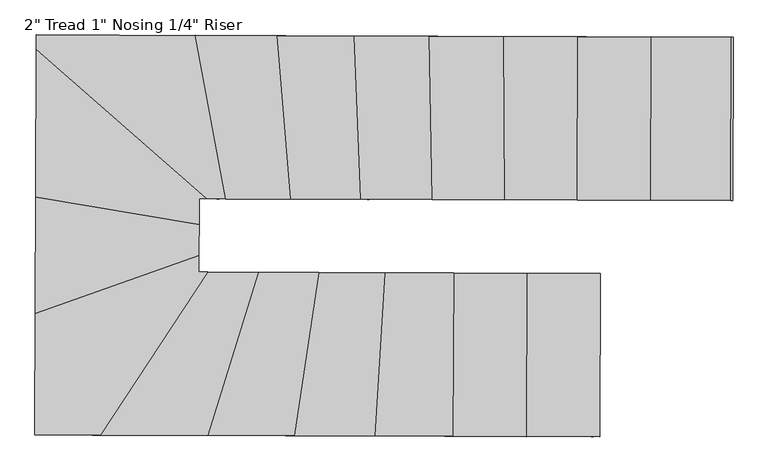
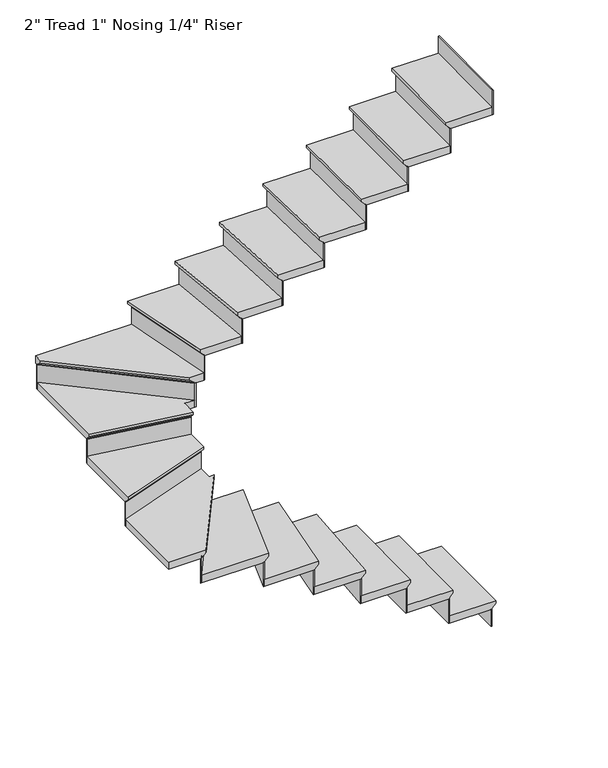
"""IFC4 building model written with IfcOpenShell, lengths in millimetres: stair flight geometry."""

from ifc_helpers import new_model, si_unit, origin, place, context, project, spatial, faceted_brep, source, transform, mapped, element, save


def stair_flight_0ba6b5c4(model_context):
    return source(origin(), model_context, "Body", "Brep", [
        faceted_brep([(-2339.9228929, -4204.0248458, 150.2833333), (-2339.9228929, -4204.0248458, 169.3333333), (-2342.0274141, -4826.0015756, 169.3333333), (-2342.0274141, -4826.0015756, 150.2833333), (-2365.3227475, -4203.9389029, 124.8833333), (-2367.4272687, -4825.9156326, 124.8833333), (-2644.7211481, -4202.9935301, 169.3333333), (-2646.8256693, -4824.9702599, 169.3333333), (-2367.4272687, -4825.9156326, 118.5333333), (-2646.8256693, -4824.9702599, 118.5333333), (-2644.7211481, -4202.9935301, 118.5333333), (-2365.3227475, -4203.9389029, 118.5333333)], [[[0, 1, 2, 3]], [[4, 0, 3, 5]], [[2, 1, 6, 7]], [[8, 9, 10, 11]], [[2, 7, 9, 8, 5, 3]], [[8, 11, 4, 5]], [[6, 1, 0, 4, 11, 10]], [[7, 6, 10, 9]]]),
        faceted_brep([(-2365.3227475, -4203.9389029, 118.5333333), (-2365.3227475, -4203.9389029, 0.0), (-2371.6727112, -4203.9174171, 0.0), (-2371.6727112, -4203.9174171, 118.5333333), (-2367.4272687, -4825.9156326, 118.5333333), (-2373.7772323, -4825.8941469, 118.5333333), (-2373.7772323, -4825.8941469, 0.0), (-2367.4272687, -4825.9156326, 0.0)], [[[0, 1, 2, 3]], [[4, 5, 6, 7]], [[1, 0, 4, 7]], [[2, 1, 7, 6]], [[3, 2, 6, 5]], [[0, 3, 5, 4]]]),
        faceted_brep([(-2644.7211481, -4202.9935301, 287.8666667), (-2644.7211481, -4202.9935301, 118.5333333), (-2651.0711118, -4202.9720444, 118.5333333), (-2651.0711118, -4202.9720444, 287.8666667), (-2646.8256693, -4824.9702599, 287.8666667), (-2653.175633, -4824.9487741, 287.8666667), (-2653.175633, -4824.9487741, 118.5333333), (-2646.8256693, -4824.9702599, 118.5333333)], [[[0, 1, 2, 3]], [[4, 5, 6, 7]], [[1, 0, 4, 7]], [[2, 1, 7, 6]], [[3, 2, 6, 5]], [[0, 3, 5, 4]]]),
        faceted_brep([(-2621.4258147, -4825.0562028, 338.6666667), (-2619.3212935, -4203.0794731, 338.6666667), (-2924.1195488, -4202.0481574, 338.6666667), (-2926.2240699, -4824.0248871, 338.6666667), (-2646.8256693, -4824.9702599, 287.8666667), (-2926.2240699, -4824.0248871, 287.8666667), (-2924.1195488, -4202.0481574, 287.8666667), (-2644.7211481, -4202.9935301, 287.8666667), (-2646.8256693, -4824.9702599, 294.2166667), (-2621.4258147, -4825.0562028, 319.6166667), (-2644.7211481, -4202.9935301, 294.2166667), (-2619.3212935, -4203.0794731, 319.6166667)], [[[0, 1, 2, 3]], [[4, 5, 6, 7]], [[0, 3, 5, 4, 8, 9]], [[4, 7, 10, 8]], [[2, 1, 11, 10, 7, 6]], [[3, 2, 6, 5]], [[11, 1, 0, 9]], [[10, 11, 9, 8]]]),
        faceted_brep([(-2924.1195488, -4202.0481574, 457.2), (-2924.1195488, -4202.0481574, 287.8666667), (-2930.4695124, -4202.0266716, 287.8666667), (-2930.4695124, -4202.0266716, 457.2), (-2926.2240699, -4824.0248871, 457.2), (-2932.5740336, -4824.0034014, 457.2), (-2932.5740336, -4824.0034014, 287.8666667), (-2926.2240699, -4824.0248871, 287.8666667)], [[[0, 1, 2, 3]], [[4, 5, 6, 7]], [[1, 0, 4, 7]], [[2, 1, 7, 6]], [[3, 2, 6, 5]], [[0, 3, 5, 4]]]),
        faceted_brep([(-2900.8242153, -4824.1108301, 508.0), (-2898.7196941, -4202.1341003, 508.0), (-3185.4282049, -4201.1639931, 508.0), (-3223.7984946, -4823.0180139, 508.0), (-2926.2240699, -4824.0248871, 457.2), (-3223.7984946, -4823.0180139, 457.2), (-3185.4282049, -4201.1639931, 457.2), (-2924.1195488, -4202.0481574, 457.2), (-2926.2240699, -4824.0248871, 463.55), (-2900.8242153, -4824.1108301, 488.95), (-2924.1195488, -4202.0481574, 463.55), (-2898.7196941, -4202.1341003, 488.95)], [[[0, 1, 2, 3]], [[4, 5, 6, 7]], [[0, 3, 5, 4, 8, 9]], [[4, 7, 10, 8]], [[2, 1, 11, 10, 7, 6]], [[3, 2, 6, 5]], [[11, 1, 0, 9]], [[10, 11, 9, 8]]]),
        faceted_brep([(-3185.4282049, -4201.1639931, 626.5333333), (-3185.4282049, -4201.1639931, 457.2), (-3191.7889535, -4201.1424708, 457.2), (-3191.7889535, -4201.1424708, 626.5333333), (-3223.7984946, -4823.0180139, 626.5333333), (-3230.1592432, -4822.9964917, 626.5333333), (-3230.1592432, -4822.9964917, 457.2), (-3223.7984946, -4823.0180139, 457.2)], [[[0, 1, 2, 3]], [[4, 5, 6, 7]], [[1, 0, 4, 7]], [[2, 1, 7, 6]], [[3, 2, 6, 5]], [[0, 3, 5, 4]]]),
        faceted_brep([(-3198.3555003, -4823.1041029, 677.3333333), (-3159.9852105, -4201.250082, 677.3333333), (-3437.1491731, -4200.3122697, 677.3333333), (-3531.3418182, -4821.97741, 677.3333333), (-3223.7984946, -4823.0180139, 626.5333333), (-3531.3418182, -4821.97741, 626.5333333), (-3437.1491731, -4200.3122697, 626.5333333), (-3185.4282049, -4201.1639931, 626.5333333), (-3223.7984946, -4823.0180139, 632.8833333), (-3198.3555003, -4823.1041029, 658.2833333), (-3185.4282049, -4201.1639931, 632.8833333), (-3159.9852105, -4201.250082, 658.2833333)], [[[0, 1, 2, 3]], [[4, 5, 6, 7]], [[0, 3, 5, 4, 8, 9]], [[4, 7, 10, 8]], [[2, 1, 11, 10, 7, 6]], [[3, 2, 6, 5]], [[11, 1, 0, 9]], [[10, 11, 9, 8]]]),
        faceted_brep([(-3437.1491731, -4200.3122697, 795.8666667), (-3437.1491731, -4200.3122697, 626.5333333), (-3443.568358, -4200.2905498, 626.5333333), (-3443.568358, -4200.2905498, 795.8666667), (-3531.3418182, -4821.97741, 795.8666667), (-3537.7610031, -4821.95569, 795.8666667), (-3537.7610031, -4821.95569, 626.5333333), (-3531.3418182, -4821.97741, 626.5333333)], [[[0, 1, 2, 3]], [[4, 5, 6, 7]], [[1, 0, 4, 7]], [[2, 1, 7, 6]], [[3, 2, 6, 5]], [[0, 3, 5, 4]]]),
        faceted_brep([(-3505.6650785, -4822.0642898, 846.6666667), (-3411.4724335, -4200.3991496, 846.6666667), (-3668.9000376, -4199.5281172, 846.6666667), (-3860.1305452, -4820.8649201, 846.6666667), (-3531.3418182, -4821.97741, 795.8666667), (-3860.1305452, -4820.8649201, 795.8666667), (-3668.9000376, -4199.5281172, 795.8666667), (-3437.1491731, -4200.3122697, 795.8666667), (-3531.3418182, -4821.97741, 802.2166667), (-3505.6650785, -4822.0642898, 827.6166667), (-3437.1491731, -4200.3122697, 802.2166667), (-3411.4724335, -4200.3991496, 827.6166667)], [[[0, 1, 2, 3]], [[4, 5, 6, 7]], [[0, 3, 5, 4, 8, 9]], [[4, 7, 10, 8]], [[2, 1, 11, 10, 7, 6]], [[3, 2, 6, 5]], [[11, 1, 0, 9]], [[10, 11, 9, 8]]]),
        faceted_brep([(-3668.9000376, -4199.5281172, 965.2), (-3668.9000376, -4199.5281172, 795.8666667), (-3675.5370713, -4199.5056601, 795.8666667), (-3675.5370713, -4199.5056601, 965.2), (-3860.1305452, -4820.8649201, 965.2), (-3866.7675788, -4820.842463, 965.2), (-3866.7675788, -4820.842463, 795.8666667), (-3860.1305452, -4820.8649201, 795.8666667)], [[[0, 1, 2, 3]], [[4, 5, 6, 7]], [[1, 0, 4, 7]], [[2, 1, 7, 6]], [[3, 2, 6, 5]], [[0, 3, 5, 4]]]),
        faceted_brep([(-3833.5824104, -4820.9547484, 1016.0), (-3642.3519028, -4199.6179455, 1016.0), (-3864.4957991, -4198.8662992, 1016.0), (-4274.0422035, -4819.4644081, 1016.0), (-3860.1305452, -4820.8649201, 965.2), (-4274.0422035, -4819.4644081, 965.2), (-3864.4957991, -4198.8662992, 965.2), (-3668.9000376, -4199.5281172, 965.2), (-3860.1305452, -4820.8649201, 971.55), (-3833.5824104, -4820.9547484, 996.95), (-3668.9000376, -4199.5281172, 971.55), (-3642.3519028, -4199.6179455, 996.95)], [[[0, 1, 2, 3]], [[4, 5, 6, 7]], [[0, 3, 5, 4, 8, 9]], [[4, 7, 10, 8]], [[2, 1, 11, 10, 7, 6]], [[3, 2, 6, 5]], [[11, 1, 0, 9]], [[10, 11, 9, 8]]]),
        faceted_brep([(-3864.4957991, -4198.8662992, 1134.5333333), (-3864.4957991, -4198.8662992, 965.2), (-3872.0869257, -4198.8406138, 965.2), (-3872.0869257, -4198.8406138, 1134.5333333), (-4274.0422035, -4819.4644081, 1134.5333333), (-4281.6333301, -4819.4387227, 1134.5333333), (-4281.6333301, -4819.4387227, 965.2), (-4274.0422035, -4819.4644081, 965.2)], [[[0, 1, 2, 3]], [[4, 5, 6, 7]], [[1, 0, 4, 7]], [[2, 1, 7, 6]], [[3, 2, 6, 5]], [[0, 3, 5, 4]]]),
        faceted_brep([(-4490.0684734, -4328.5349965, 1185.3333333), (-4491.7270905, -4818.7278493, 1185.3333333), (-4243.677697, -4819.5671495, 1185.3333333), (-3834.1312926, -4198.9690405, 1185.3333333), (-3867.6458395, -4198.8556407, 1185.3333333), (-3867.338948, -4108.1559559, 1185.3333333), (-4491.7270905, -4818.7278493, 1134.5333333), (-4490.0684734, -4328.5349965, 1134.5333333), (-3867.338948, -4108.1559559, 1134.5333333), (-3867.6458395, -4198.8556407, 1134.5333333), (-3864.4957991, -4198.8662992, 1134.5333333), (-4274.0422035, -4819.4644081, 1134.5333333), (-4274.0422035, -4819.4644081, 1140.8833333), (-4243.677697, -4819.5671495, 1166.2833333), (-3864.4957991, -4198.8662992, 1140.8833333), (-3834.1312926, -4198.9690405, 1166.2833333)], [[[0, 1, 2, 3, 4, 5]], [[6, 7, 8, 9, 10, 11]], [[1, 0, 7, 6]], [[2, 1, 6, 11, 12, 13]], [[11, 10, 14, 12]], [[4, 3, 15, 14, 10, 9]], [[5, 4, 9, 8]], [[0, 5, 8, 7]], [[15, 3, 2, 13]], [[14, 15, 13, 12]]]),
        faceted_brep([(-3867.338948, -4108.1559559, 1303.8666667), (-3867.338948, -4108.1559559, 1134.5333333), (-3867.316129, -4101.4119712, 1134.5333333), (-3867.316129, -4101.4119712, 1303.8666667), (-4490.0684734, -4328.5349965, 1303.8666667), (-4490.0456544, -4321.7910118, 1303.8666667), (-4490.0456544, -4321.7910118, 1134.5333333), (-4490.0684734, -4328.5349965, 1134.5333333)], [[[0, 1, 2, 3]], [[4, 5, 6, 7]], [[1, 0, 4, 7]], [[2, 1, 7, 6]], [[3, 2, 6, 5]], [[0, 3, 5, 4]]]),
        faceted_brep([(-4490.1597492, -4355.5109354, 1354.6666667), (-3867.4302238, -4135.1318948, 1354.6666667), (-3866.9449143, -3991.702012, 1354.6666667), (-4488.5718319, -3886.2129338, 1354.6666667), (-4490.0684734, -4328.5349965, 1303.8666667), (-4488.5718319, -3886.2129338, 1303.8666667), (-3866.9449143, -3991.702012, 1303.8666667), (-3867.338948, -4108.1559559, 1303.8666667), (-4490.0684734, -4328.5349965, 1310.2166667), (-4490.1597492, -4355.5109354, 1335.6166667), (-3867.338948, -4108.1559559, 1310.2166667), (-3867.4302238, -4135.1318948, 1335.6166667)], [[[0, 1, 2, 3]], [[4, 5, 6, 7]], [[0, 3, 5, 4, 8, 9]], [[4, 7, 10, 8]], [[3, 2, 6, 5]], [[11, 1, 0, 9]], [[10, 11, 9, 8]], [[2, 1, 11, 10, 7, 6]]]),
        faceted_brep([(-3866.9449143, -3991.702012, 1473.2), (-3866.9449143, -3991.702012, 1303.8666667), (-3866.9231337, -3985.2649249, 1303.8666667), (-3866.9231337, -3985.2649249, 1473.2), (-4488.5718319, -3886.2129338, 1473.2), (-4488.5500514, -3879.7758467, 1473.2), (-4488.5500514, -3879.7758467, 1303.8666667), (-4488.5718319, -3886.2129338, 1303.8666667)], [[[0, 1, 2, 3]], [[4, 5, 6, 7]], [[1, 0, 4, 7]], [[2, 1, 7, 6]], [[3, 2, 6, 5]], [[0, 3, 5, 4]]]),
        faceted_brep([(-4488.6589541, -3911.9612823, 1524.0), (-3867.0320364, -4017.4503605, 1524.0), (-3866.7004668, -3919.4572401, 1524.0), (-3799.1127501, -3919.6859299, 1524.0), (-4486.6423896, -3315.9795656, 1524.0), (-4488.5718319, -3886.2129338, 1473.2), (-4486.6423896, -3315.9795656, 1473.2), (-3799.1127501, -3919.6859299, 1473.2), (-3866.7004668, -3919.4572401, 1473.2), (-3866.9449143, -3991.702012, 1473.2), (-4488.5718319, -3886.2129338, 1479.55), (-4488.6589541, -3911.9612823, 1504.95), (-3866.9449143, -3991.702012, 1479.55), (-3867.0320364, -4017.4503605, 1504.95)], [[[0, 1, 2, 3, 4]], [[5, 6, 7, 8, 9]], [[0, 4, 6, 5, 10, 11]], [[5, 9, 12, 10]], [[2, 1, 13, 12, 9, 8]], [[4, 3, 7, 6]], [[13, 1, 0, 11]], [[12, 13, 11, 10]], [[3, 2, 8, 7]]]),
        faceted_brep([(-3799.1127501, -3919.6859299, 1642.5333333), (-3799.1127501, -3919.6859299, 1473.2), (-3789.4516067, -3919.7186194, 1473.2), (-3789.4516067, -3919.7186194, 1642.5333333), (-4486.6423896, -3315.9795656, 1642.5333333), (-4486.613881, -3307.5540264, 1642.5333333), (-4486.613881, -3307.5540264, 1473.2), (-4486.6423896, -3315.9795656, 1473.2)], [[[0, 1, 2, 3]], [[4, 5, 6, 7]], [[1, 0, 4, 7]], [[2, 1, 7, 6]], [[3, 2, 6, 5]], [[0, 3, 5, 4]]]),
        faceted_brep([(-3855.3688773, -3297.511731, 1693.3333333), (-4486.5726753, -3295.3759891, 1693.3333333), (-4486.7564243, -3349.6817226, 1693.3333333), (-3837.757324, -3919.5551721, 1693.3333333), (-3739.9081193, -3919.8862548, 1693.3333333), (-4486.5726753, -3295.3759891, 1642.5333333), (-3855.3688773, -3297.511731, 1642.5333333), (-3739.9081193, -3919.8862548, 1642.5333333), (-3799.1127501, -3919.6859299, 1642.5333333), (-4486.6423896, -3315.9795656, 1642.5333333), (-3799.1127501, -3919.6859299, 1648.8833333), (-4486.6423896, -3315.9795656, 1648.8833333), (-3837.757324, -3919.5551721, 1674.2833333), (-4486.7564243, -3349.6817226, 1674.2833333)], [[[0, 1, 2, 3, 4]], [[5, 6, 7, 8, 9]], [[1, 0, 6, 5]], [[9, 8, 10, 11]], [[4, 3, 12, 10, 8, 7]], [[0, 4, 7, 6]], [[12, 3, 2, 13]], [[10, 12, 13, 11]], [[2, 1, 5, 9, 11, 13]]]),
        faceted_brep([(-3739.9081193, -3919.8862548, 1811.8666667), (-3739.9081193, -3919.8862548, 1642.5333333), (-3733.4457151, -3919.908121, 1642.5333333), (-3733.4457151, -3919.908121, 1811.8666667), (-3855.3688773, -3297.511731, 1811.8666667), (-3848.9064731, -3297.5335972, 1811.8666667), (-3848.9064731, -3297.5335972, 1642.5333333), (-3855.3688773, -3297.511731, 1642.5333333)], [[[0, 1, 2, 3]], [[4, 5, 6, 7]], [[1, 0, 4, 7]], [[2, 1, 7, 6]], [[3, 2, 6, 5]], [[0, 3, 5, 4]]]),
        faceted_brep([(-3881.2184941, -3297.4242662, 1862.6666667), (-3765.7577361, -3919.79879, 1862.6666667), (-3493.4024921, -3920.7203315, 1862.6666667), (-3543.7965904, -3298.5659674, 1862.6666667), (-3855.3688773, -3297.511731, 1811.8666667), (-3543.7965904, -3298.5659674, 1811.8666667), (-3493.4024921, -3920.7203315, 1811.8666667), (-3739.9081193, -3919.8862548, 1811.8666667), (-3855.3688773, -3297.511731, 1818.2166667), (-3881.2184941, -3297.4242662, 1843.6166667), (-3739.9081193, -3919.8862548, 1818.2166667), (-3765.7577361, -3919.79879, 1843.6166667)], [[[0, 1, 2, 3]], [[4, 5, 6, 7]], [[0, 3, 5, 4, 8, 9]], [[4, 7, 10, 8]], [[2, 1, 11, 10, 7, 6]], [[3, 2, 6, 5]], [[11, 1, 0, 9]], [[10, 11, 9, 8]]]),
        faceted_brep([(-3493.4024921, -3920.7203315, 1981.2), (-3493.4024921, -3920.7203315, 1811.8666667), (-3487.0299488, -3920.7418937, 1811.8666667), (-3487.0299488, -3920.7418937, 1981.2), (-3543.7965904, -3298.5659674, 1981.2), (-3537.4240471, -3298.5875295, 1981.2), (-3537.4240471, -3298.5875295, 1811.8666667), (-3543.7965904, -3298.5659674, 1811.8666667)], [[[0, 1, 2, 3]], [[4, 5, 6, 7]], [[1, 0, 4, 7]], [[2, 1, 7, 6]], [[3, 2, 6, 5]], [[0, 3, 5, 4]]]),
        faceted_brep([(-3569.2867636, -3298.4797188, 2032.0), (-3518.8926653, -3920.634083, 2032.0), (-3226.664936, -3921.622865, 2032.0), (-3251.8690415, -3299.5537338, 2032.0), (-3543.7965904, -3298.5659674, 1981.2), (-3251.8690415, -3299.5537338, 1981.2), (-3226.664936, -3921.622865, 1981.2), (-3493.4024921, -3920.7203315, 1981.2), (-3543.7965904, -3298.5659674, 1987.55), (-3569.2867636, -3298.4797188, 2012.95), (-3493.4024921, -3920.7203315, 1987.55), (-3518.8926653, -3920.634083, 2012.95)], [[[0, 1, 2, 3]], [[4, 5, 6, 7]], [[0, 3, 5, 4, 8, 9]], [[4, 7, 10, 8]], [[2, 1, 11, 10, 7, 6]], [[3, 2, 6, 5]], [[11, 1, 0, 9]], [[10, 11, 9, 8]]]),
        faceted_brep([(-3226.664936, -3921.622865, 2150.5333333), (-3226.664936, -3921.622865, 1981.2), (-3220.3088547, -3921.6443715, 1981.2), (-3220.3088547, -3921.6443715, 2150.5333333), (-3251.8690415, -3299.5537338, 2150.5333333), (-3245.5129602, -3299.5752402, 2150.5333333), (-3245.5129602, -3299.5752402, 1981.2), (-3251.8690415, -3299.5537338, 1981.2)], [[[0, 1, 2, 3]], [[4, 5, 6, 7]], [[1, 0, 4, 7]], [[2, 1, 7, 6]], [[3, 2, 6, 5]], [[0, 3, 5, 4]]]),
        faceted_brep([(-3277.2933666, -3299.467708, 2201.3333333), (-3252.0892611, -3921.5368393, 2201.3333333), (-2953.9711928, -3922.5455519, 2201.3333333), (-2965.8021755, -3300.52167, 2201.3333333), (-3251.8690415, -3299.5537338, 2150.5333333), (-2965.8021755, -3300.52167, 2150.5333333), (-2953.9711928, -3922.5455519, 2150.5333333), (-3226.664936, -3921.622865, 2150.5333333), (-3251.8690415, -3299.5537338, 2156.8833333), (-3277.2933666, -3299.467708, 2182.2833333), (-3226.664936, -3921.622865, 2156.8833333), (-3252.0892611, -3921.5368393, 2182.2833333)], [[[0, 1, 2, 3]], [[4, 5, 6, 7]], [[0, 3, 5, 4, 8, 9]], [[4, 7, 10, 8]], [[2, 1, 11, 10, 7, 6]], [[3, 2, 6, 5]], [[11, 1, 0, 9]], [[10, 11, 9, 8]]]),
        faceted_brep([(-2953.9711928, -3922.5455519, 2319.8666667), (-2953.9711928, -3922.5455519, 2150.5333333), (-2947.6196355, -3922.567043, 2150.5333333), (-2947.6196355, -3922.567043, 2319.8666667), (-2965.8021755, -3300.52167, 2319.8666667), (-2959.4506182, -3300.5431611, 2319.8666667), (-2959.4506182, -3300.5431611, 2150.5333333), (-2965.8021755, -3300.52167, 2150.5333333)], [[[0, 1, 2, 3]], [[4, 5, 6, 7]], [[1, 0, 4, 7]], [[2, 1, 7, 6]], [[3, 2, 6, 5]], [[0, 3, 5, 4]]]),
        faceted_brep([(-2991.2084046, -3300.4357054, 2370.6666667), (-2979.3774219, -3922.4595874, 2370.6666667), (-2678.7239035, -3923.476879, 2370.6666667), (-2682.2633211, -3301.4810524, 2370.6666667), (-2965.8021755, -3300.52167, 2319.8666667), (-2682.2633211, -3301.4810524, 2319.8666667), (-2678.7239035, -3923.476879, 2319.8666667), (-2953.9711928, -3922.5455519, 2319.8666667), (-2965.8021755, -3300.52167, 2326.2166667), (-2991.2084046, -3300.4357054, 2351.6166667), (-2953.9711928, -3922.5455519, 2326.2166667), (-2979.3774219, -3922.4595874, 2351.6166667)], [[[0, 1, 2, 3]], [[4, 5, 6, 7]], [[0, 3, 5, 4, 8, 9]], [[4, 7, 10, 8]], [[2, 1, 11, 10, 7, 6]], [[3, 2, 6, 5]], [[11, 1, 0, 9]], [[10, 11, 9, 8]]]),
        faceted_brep([(-2678.7239035, -3923.476879, 2489.2), (-2678.7239035, -3923.476879, 2319.8666667), (-2672.3736784, -3923.4983656, 2319.8666667), (-2672.3736784, -3923.4983656, 2489.2), (-2682.2633211, -3301.4810524, 2489.2), (-2675.913096, -3301.502539, 2489.2), (-2675.913096, -3301.502539, 2319.8666667), (-2682.2633211, -3301.4810524, 2319.8666667)], [[[0, 1, 2, 3]], [[4, 5, 6, 7]], [[1, 0, 4, 7]], [[2, 1, 7, 6]], [[3, 2, 6, 5]], [[0, 3, 5, 4]]]),
        faceted_brep([(-2707.6642214, -3301.3951058, 2540.0), (-2704.1248038, -3923.3909324, 2540.0), (-2402.148518, -3924.4126998, 2540.0), (-2400.0439968, -3302.43597, 2540.0), (-2682.2633211, -3301.4810524, 2489.2), (-2400.0439968, -3302.43597, 2489.2), (-2402.148518, -3924.4126998, 2489.2), (-2678.7239035, -3923.476879, 2489.2), (-2682.2633211, -3301.4810524, 2495.55), (-2707.6642214, -3301.3951058, 2520.95), (-2678.7239035, -3923.476879, 2495.55), (-2704.1248038, -3923.3909324, 2520.95)], [[[0, 1, 2, 3]], [[4, 5, 6, 7]], [[0, 3, 5, 4, 8, 9]], [[4, 7, 10, 8]], [[2, 1, 11, 10, 7, 6]], [[3, 2, 6, 5]], [[11, 1, 0, 9]], [[10, 11, 9, 8]]]),
        faceted_brep([(-2402.148518, -3924.4126998, 2658.5333333), (-2402.148518, -3924.4126998, 2489.2), (-2395.7985543, -3924.4341855, 2489.2), (-2395.7985543, -3924.4341855, 2658.5333333), (-2400.0439968, -3302.43597, 2658.5333333), (-2393.6940331, -3302.4574557, 2658.5333333), (-2393.6940331, -3302.4574557, 2489.2), (-2400.0439968, -3302.43597, 2489.2)], [[[0, 1, 2, 3]], [[4, 5, 6, 7]], [[1, 0, 4, 7]], [[2, 1, 7, 6]], [[3, 2, 6, 5]], [[0, 3, 5, 4]]]),
        faceted_brep([(-2425.4438514, -3302.350027, 2709.3333333), (-2427.5483726, -3924.3267568, 2709.3333333), (-2122.7501174, -3925.3580725, 2709.3333333), (-2120.6455962, -3303.3813428, 2709.3333333), (-2400.0439968, -3302.43597, 2658.5333333), (-2120.6455962, -3303.3813428, 2658.5333333), (-2122.7501174, -3925.3580725, 2658.5333333), (-2402.148518, -3924.4126998, 2658.5333333), (-2400.0439968, -3302.43597, 2664.8833333), (-2425.4438514, -3302.350027, 2690.2833333), (-2402.148518, -3924.4126998, 2664.8833333), (-2427.5483726, -3924.3267568, 2690.2833333)], [[[0, 1, 2, 3]], [[4, 5, 6, 7]], [[0, 3, 5, 4, 8, 9]], [[4, 7, 10, 8]], [[2, 1, 11, 10, 7, 6]], [[3, 2, 6, 5]], [[11, 1, 0, 9]], [[10, 11, 9, 8]]]),
        faceted_brep([(-2122.7501174, -3925.3580725, 2827.8666667), (-2122.7501174, -3925.3580725, 2658.5333333), (-2116.4001537, -3925.3795583, 2658.5333333), (-2116.4001537, -3925.3795583, 2827.8666667), (-2120.6455962, -3303.3813428, 2827.8666667), (-2114.2956325, -3303.4028285, 2827.8666667), (-2114.2956325, -3303.4028285, 2658.5333333), (-2120.6455962, -3303.3813428, 2658.5333333)], [[[0, 1, 2, 3]], [[4, 5, 6, 7]], [[1, 0, 4, 7]], [[2, 1, 7, 6]], [[3, 2, 6, 5]], [[0, 3, 5, 4]]]),
        faceted_brep([(-1843.3517167, -3926.3034453, 2997.2), (-1843.3517167, -3926.3034453, 2827.8666667), (-1837.0017531, -3926.324931, 2827.8666667), (-1837.0017531, -3926.324931, 2997.2), (-1841.2471955, -3304.3267155, 2997.2), (-1834.8972319, -3304.3482013, 2997.2), (-1834.8972319, -3304.3482013, 2827.8666667), (-1841.2471955, -3304.3267155, 2827.8666667)], [[[0, 1, 2, 3]], [[4, 5, 6, 7]], [[1, 0, 4, 7]], [[2, 1, 7, 6]], [[3, 2, 6, 5]], [[0, 3, 5, 4]]]),
        faceted_brep([(-2146.0454508, -3303.2953998, 2878.6666667), (-2148.149972, -3925.2721295, 2878.6666667), (-1843.3517167, -3926.3034453, 2878.6666667), (-1841.2471955, -3304.3267155, 2878.6666667), (-2120.6455962, -3303.3813428, 2827.8666667), (-1841.2471955, -3304.3267155, 2827.8666667), (-1843.3517167, -3926.3034453, 2827.8666667), (-2122.7501174, -3925.3580725, 2827.8666667), (-2120.6455962, -3303.3813428, 2834.2166667), (-2146.0454508, -3303.2953998, 2859.6166667), (-2122.7501174, -3925.3580725, 2834.2166667), (-2148.149972, -3925.2721295, 2859.6166667)], [[[0, 1, 2, 3]], [[4, 5, 6, 7]], [[0, 3, 5, 4, 8, 9]], [[4, 7, 10, 8]], [[2, 1, 11, 10, 7, 6]], [[3, 2, 6, 5]], [[11, 1, 0, 9]], [[10, 11, 9, 8]]]),
    ])


if __name__ == "__main__":
    model = new_model("IFC4")
    model_context = context("Model", 3, world=origin())
    ifc_project = project(units=[si_unit("LENGTHUNIT", "METRE", prefix="MILLI")], contexts=[model_context])
    site = spatial("IfcSite", under=ifc_project)
    building = spatial("IfcBuilding", under=site)
    placement = place(None, origin())
    stair_flight_shape = stair_flight_0ba6b5c4(model_context)
    element("IfcStairFlight", 1, ObjectType="2\" Tread 1\" Nosing 1/4\" Riser", at=placement, inside=building, context=model_context, shape_type="MappedRepresentation", body=[
        mapped(stair_flight_shape, transform((0.0, 0.0, 0.0), x_axis=(1.0, 0.0, 0.0), y_axis=(0.0, 1.0, 0.0), z_axis=(0.0, 0.0, 1.0))),
    ])
    save(model, "model.ifc")
